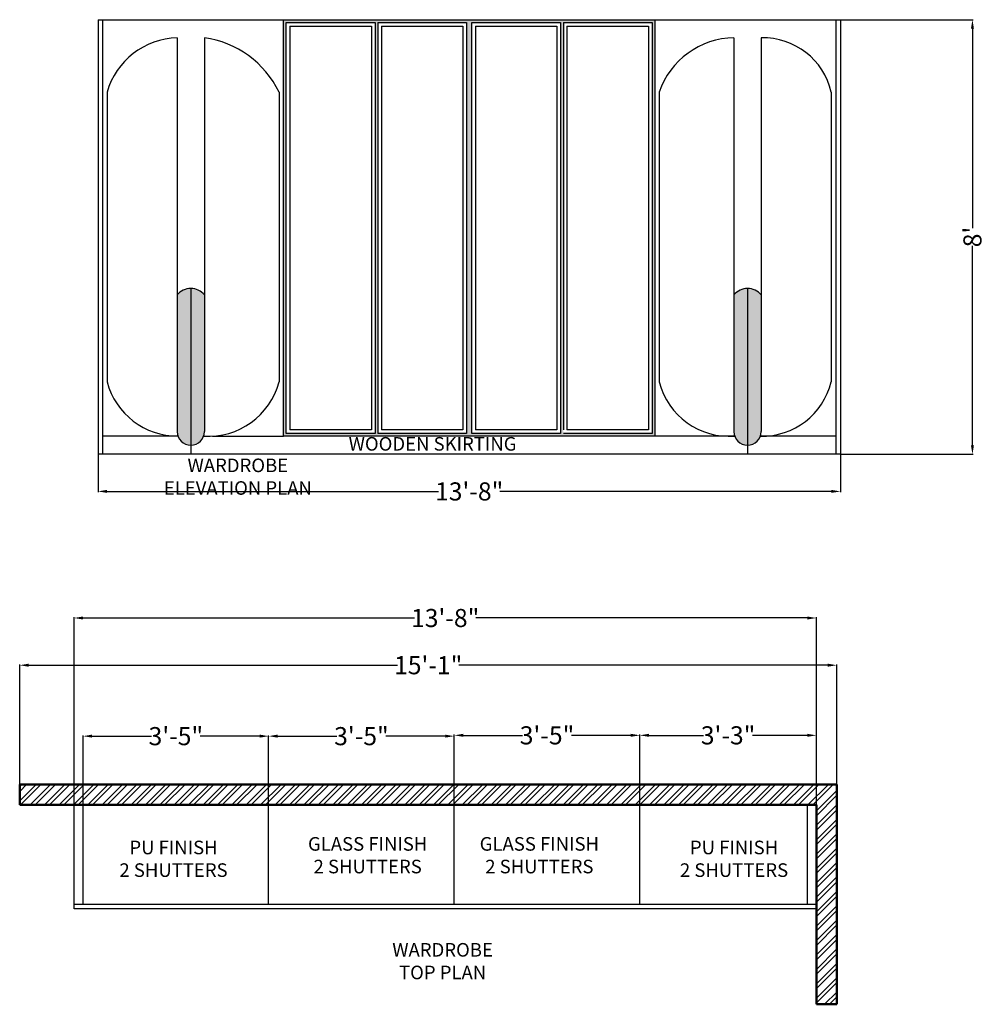
# Model space of a CAD drawing. Units: inches. Extents: x 210 to 423, y 38 to 255.
import ezdxf

# ---------------------------------------------------------------- set-up
doc = ezdxf.new("R2010")
doc.units = ezdxf.units.IN
doc.header["$MEASUREMENT"] = 0
for name, color, linetype, lineweight in [('A-ANNO-DIMS', 2, 'Continuous', 18), ('A-ANNO-TEXT', 7, 'Continuous', 18), ('A-FURN', 7, 'Continuous', 25), ('A-FURN-PATT', 42, 'Continuous', 13), ('A-WALL', 1, 'Continuous', 50), ('A-WALL-PATT', 8, 'Continuous', 13)]:
    doc.layers.add(name, color=color, linetype=linetype, lineweight=lineweight)
doc.styles.get("Standard").update_dxf_attribs({"font": 'arial.ttf'})
doc.dimstyles.get("Standard").update_dxf_attribs({"dimtxt": 4, "dimasz": 2, "dimexe": 0.18, "dimexo": 0.0625, "dimgap": 0.09, "dimtad": 0, "dimdec": 0, "dimzin": 0, "dimdsep": 46, "dimlunit": 4, "dimtxsty": 'Standard', "dimcen": 0.09, "dimadec": 0, "dimazin": 0, "dimtfac": 1, "dimtdec": 0, "dimtofl": 0, "dimtmove": 0, "dimatfit": 3, "dimfxl": 1, "dimtolj": 1, "dimtzin": 0, "dimarcsym": 0})

# ---------------------------------------------------------------- blocks, each defined once
blk = doc.blocks.new('*D1')
at = {"layer": 'A-ANNO-DIMS', "color": 0, "lineweight": -2, "transparency": 16777216}
for p, q in [((227.24, 159.18), (227.24, 150.86)), ((391.24, 159.18), (391.24, 150.86)), ((229.24, 151.04), (302.47, 151.04)), ((389.24, 151.04), (316.01, 151.04))]:
    blk.add_line(p, q, dxfattribs=at)
at = {"layer": 'A-ANNO-DIMS', "color": 0, "transparency": 16777216}
for points in [[(229.24, 151.38), (229.24, 150.71), (227.24, 151.04)], [(389.24, 151.38), (389.24, 150.71), (391.24, 151.04)]]:
    blk.add_solid(points, dxfattribs=at)
at = {"layer": 'Defpoints', "color": 0, "transparency": 16777216}
for p in [(227.24, 159.24), (391.24, 159.24), (227.24, 151.04)]:
    blk.add_point(p, dxfattribs=at)
at = {"layer": 'A-ANNO-DIMS', "color": 0, "transparency": 16777216, "insert": (309.24, 151.04), "char_height": 4, "attachment_point": 5}
blk.add_mtext('\\A1;13\'-8"', dxfattribs=at)
blk = doc.blocks.new('*D2')
at = {"layer": 'A-ANNO-DIMS', "color": 0, "lineweight": -2, "transparency": 16777216}
for p, q in [((391.3, 255.24), (420.6, 255.24)), ((420.42, 253.24), (420.42, 209.18)), ((420.42, 161.24), (420.42, 205.31)), ((391.3, 159.24), (420.6, 159.24))]:
    blk.add_line(p, q, dxfattribs=at)
at = {"layer": 'A-ANNO-DIMS', "color": 0, "transparency": 16777216}
for points in [[(420.08, 253.24), (420.75, 253.24), (420.42, 255.24)], [(420.08, 161.24), (420.75, 161.24), (420.42, 159.24)]]:
    blk.add_solid(points, dxfattribs=at)
at = {"layer": 'Defpoints', "color": 0, "transparency": 16777216}
for p in [(391.24, 255.24), (420.42, 255.24), (391.24, 159.24)]:
    blk.add_point(p, dxfattribs=at)
at = {"layer": 'A-ANNO-DIMS', "color": 0, "transparency": 16777216, "insert": (420.42, 207.24), "char_height": 4, "attachment_point": 5, "rotation": 90}
blk.add_mtext("\\A1;8'", dxfattribs=at)
blk = doc.blocks.new('*D3')
at = {"layer": 'A-ANNO-DIMS', "color": 0, "lineweight": -2, "transparency": 16777216}
for p, q in [((223.94, 81.86), (223.94, 97.16)), ((225.94, 96.98), (239.03, 96.98)), ((262.94, 96.98), (249.84, 96.98)), ((264.94, 81.86), (264.94, 97.16))]:
    blk.add_line(p, q, dxfattribs=at)
at = {"layer": 'A-ANNO-DIMS', "color": 0, "transparency": 16777216}
for points in [[(225.94, 97.32), (225.94, 96.65), (223.94, 96.98)], [(262.94, 97.32), (262.94, 96.65), (264.94, 96.98)]]:
    blk.add_solid(points, dxfattribs=at)
at = {"layer": 'Defpoints', "color": 0, "transparency": 16777216}
for p in [(264.94, 96.98), (223.94, 81.8), (264.94, 81.8)]:
    blk.add_point(p, dxfattribs=at)
at = {"layer": 'A-ANNO-DIMS', "color": 0, "transparency": 16777216, "insert": (244.44, 96.98), "char_height": 4, "attachment_point": 5}
blk.add_mtext('\\A1;3\'-5"', dxfattribs=at)
blk = doc.blocks.new('*D4')
at = {"layer": 'A-ANNO-DIMS', "color": 0, "lineweight": -2, "transparency": 16777216}
for p, q in [((264.94, 81.86), (264.94, 97.16)), ((266.94, 96.98), (280.03, 96.98)), ((303.94, 96.98), (290.84, 96.98)), ((305.94, 81.86), (305.94, 97.16))]:
    blk.add_line(p, q, dxfattribs=at)
at = {"layer": 'A-ANNO-DIMS', "color": 0, "transparency": 16777216}
for points in [[(266.94, 97.32), (266.94, 96.65), (264.94, 96.98)], [(303.94, 97.32), (303.94, 96.65), (305.94, 96.98)]]:
    blk.add_solid(points, dxfattribs=at)
at = {"layer": 'Defpoints', "color": 0, "transparency": 16777216}
for p in [(305.94, 96.98), (264.94, 81.8), (305.94, 81.8)]:
    blk.add_point(p, dxfattribs=at)
at = {"layer": 'A-ANNO-DIMS', "color": 0, "transparency": 16777216, "insert": (285.44, 96.98), "char_height": 4, "attachment_point": 5}
blk.add_mtext('\\A1;3\'-5"', dxfattribs=at)
blk = doc.blocks.new('*D5')
at = {"layer": 'A-ANNO-DIMS', "color": 0, "lineweight": -2, "transparency": 16777216}
for p, q in [((305.94, 81.86), (305.94, 97.34)), ((307.94, 97.16), (321.03, 97.16)), ((344.94, 97.16), (331.84, 97.16)), ((346.94, 81.86), (346.94, 97.34))]:
    blk.add_line(p, q, dxfattribs=at)
at = {"layer": 'A-ANNO-DIMS', "color": 0, "transparency": 16777216}
for points in [[(307.94, 97.5), (307.94, 96.83), (305.94, 97.16)], [(344.94, 97.5), (344.94, 96.83), (346.94, 97.16)]]:
    blk.add_solid(points, dxfattribs=at)
at = {"layer": 'Defpoints', "color": 0, "transparency": 16777216}
for p in [(346.94, 97.16), (305.94, 81.8), (346.94, 81.8)]:
    blk.add_point(p, dxfattribs=at)
at = {"layer": 'A-ANNO-DIMS', "color": 0, "transparency": 16777216, "insert": (326.44, 97.16), "char_height": 4, "attachment_point": 5}
blk.add_mtext('\\A1;3\'-5"', dxfattribs=at)
blk = doc.blocks.new('*D6')
at = {"layer": 'A-ANNO-DIMS', "color": 0, "lineweight": -2, "transparency": 16777216}
for p, q in [((346.94, 81.86), (346.94, 97.34)), ((348.94, 97.16), (361.03, 97.16)), ((383.94, 97.16), (371.84, 97.16)), ((385.94, 81.86), (385.94, 97.34))]:
    blk.add_line(p, q, dxfattribs=at)
at = {"layer": 'A-ANNO-DIMS', "color": 0, "transparency": 16777216}
for points in [[(348.94, 97.5), (348.94, 96.83), (346.94, 97.16)], [(383.94, 97.5), (383.94, 96.83), (385.94, 97.16)]]:
    blk.add_solid(points, dxfattribs=at)
at = {"layer": 'Defpoints', "color": 0, "transparency": 16777216}
for p in [(385.94, 97.16), (346.94, 81.8), (385.94, 81.8)]:
    blk.add_point(p, dxfattribs=at)
at = {"layer": 'A-ANNO-DIMS', "color": 0, "transparency": 16777216, "insert": (366.44, 97.16), "char_height": 4, "attachment_point": 5}
blk.add_mtext('\\A1;3\'-3"', dxfattribs=at)
blk = doc.blocks.new('*D7')
at = {"layer": 'A-ANNO-DIMS', "color": 0, "lineweight": -2, "transparency": 16777216}
for p, q in [((221.94, 58.86), (221.94, 123.26)), ((223.94, 123.08), (297.17, 123.08)), ((383.94, 123.08), (310.71, 123.08)), ((385.94, 58.86), (385.94, 123.26))]:
    blk.add_line(p, q, dxfattribs=at)
at = {"layer": 'A-ANNO-DIMS', "color": 0, "transparency": 16777216}
for points in [[(223.94, 123.41), (223.94, 122.74), (221.94, 123.08)], [(383.94, 123.41), (383.94, 122.74), (385.94, 123.08)]]:
    blk.add_solid(points, dxfattribs=at)
at = {"layer": 'Defpoints', "color": 0, "transparency": 16777216}
for p in [(221.94, 123.08), (221.94, 58.8), (385.94, 58.8)]:
    blk.add_point(p, dxfattribs=at)
at = {"layer": 'A-ANNO-DIMS', "color": 0, "transparency": 16777216, "insert": (303.94, 123.08), "char_height": 4, "attachment_point": 5}
blk.add_mtext('\\A1;13\'-8"', dxfattribs=at)
blk = doc.blocks.new('*D8')
at = {"layer": 'A-ANNO-DIMS', "color": 0, "lineweight": -2, "transparency": 16777216}
for p, q in [((209.94, 86.36), (209.94, 112.83)), ((211.94, 112.65), (293.42, 112.65)), ((388.44, 112.65), (306.96, 112.65)), ((390.44, 86.36), (390.44, 112.83))]:
    blk.add_line(p, q, dxfattribs=at)
at = {"layer": 'A-ANNO-DIMS', "color": 0, "transparency": 16777216}
for points in [[(211.94, 112.99), (211.94, 112.32), (209.94, 112.65)], [(388.44, 112.99), (388.44, 112.32), (390.44, 112.65)]]:
    blk.add_solid(points, dxfattribs=at)
at = {"layer": 'Defpoints', "color": 0, "transparency": 16777216}
for p in [(390.44, 112.65), (209.94, 86.3), (390.44, 86.3)]:
    blk.add_point(p, dxfattribs=at)
at = {"layer": 'A-ANNO-DIMS', "color": 0, "transparency": 16777216, "insert": (300.19, 112.65), "char_height": 4, "attachment_point": 5}
blk.add_mtext('\\A1;15\'-1"', dxfattribs=at)
blk = doc.blocks.new('GLASS-SHUTTER-PANEL')
for p, q in [((0, 89.2), (0, 0)), ((0, 89.2), (18, 89.2)), ((18, 89.2), (18, 0)), ((18, 0), (0, 0))]:
    blk.add_line(p, q)

msp = doc.modelspace()

# ---------------------------------------------------------------- hatches: boundary and pattern name
at = {"layer": 'A-FURN-PATT'}
h = msp.add_hatch(color=256, dxfattribs=at)
h.dxf.hatch_style = 1
h.paths.add_polyline_path([(350.24, 255.24), (309.24, 255.24), (268.24, 255.24), (268.24, 163.24), (350.24, 163.24)])
h.paths.add_polyline_path([(308.64, 163.84), (268.84, 163.84), (268.84, 254.64), (308.64, 254.64)], flags=16)
h.paths.add_polyline_path([(309.84, 254.64), (349.64, 254.64), (349.64, 163.84), (309.84, 163.84)], flags=16)
h.paths.add_polyline_path([(307.84, 253.84), (307.84, 164.64), (269.64, 164.64), (269.64, 253.84)], flags=0)
h.paths.add_polyline_path([(310.64, 253.84), (348.84, 253.84), (348.84, 164.64), (310.64, 164.64)], flags=0)
h = msp.add_hatch(color=256, dxfattribs=at)
h.dxf.hatch_style = 1
h.paths.add_polyline_path([(289.04, 254.64), (288.44, 254.64), (288.44, 163.84), (289.04, 163.84)])
h = msp.add_hatch(color=256, dxfattribs=at)
h.dxf.hatch_style = 1
h.paths.add_polyline_path([(330.04, 254.64), (329.44, 254.64), (329.44, 163.84), (330.04, 163.84)])
h = msp.add_hatch(color=256, dxfattribs=at)
h.dxf.hatch_style = 1
h.paths.add_polyline_path([(247.74, 195.86, 0.225589), (244.74, 194.43), (244.74, 164.25, 0.414214), (247.74, 161.25)])
h.paths.add_polyline_path([(250.74, 194.43, 0.225589), (247.74, 195.86), (247.74, 161.25, 0.414214), (250.74, 164.25)])
h.paths.add_polyline_path([(370.74, 195.86, 0.225589), (367.74, 194.43), (367.74, 164.25, 0.414214), (370.74, 161.25)])
h.paths.add_polyline_path([(373.74, 194.43, 0.225589), (370.74, 195.86), (370.74, 161.25, 0.414214), (373.74, 164.25)])
at = {"layer": 'A-WALL-PATT'}
h = msp.add_hatch(dxfattribs=at)
h.set_pattern_fill('ANSI32', color=256, scale=6)
h.paths.add_polyline_path([(390.44, 86.3), (385.94, 86.3), (209.94, 86.3), (209.94, 81.8), (385.94, 81.8), (385.94, 37.75), (390.44, 37.75)])

# ---------------------------------------------------------------- linework, layer by layer
at = {"layer": 'A-FURN'}
for p, q in [((227.24, 255.24), (227.24, 159.24)), ((227.24, 255.24), (268.24, 255.24)), ((228.24, 255.24), (228.24, 159.24)), ((288.44, 254.64), (288.44, 163.84)), ((289.04, 254.64), (289.04, 163.84)), ((329.44, 254.64), (329.44, 163.84)), ((330.04, 254.64), (330.04, 164.64)), ((350.24, 255.24), (391.24, 255.24)), ((390.24, 255.24), (390.24, 159.24)), ((391.24, 255.24), (391.24, 159.24)), ((288.44, 253.84), (288.44, 164.64)), ((244.74, 251.24), (244.74, 164.25)), ((250.74, 251.24), (250.74, 164.25)), ((367.74, 251.24), (367.74, 164.25)), ((373.74, 251.24), (373.74, 164.25)), ((229.24, 239.24), (229.24, 175.24)), ((267.24, 239.24), (267.24, 175.24)), ((351.24, 239.24), (351.24, 175.24)), ((389.24, 239.24), (389.24, 175.24)), ((247.74, 195.86), (247.74, 159.24)), ((370.74, 195.86), (370.74, 159.24)), ((244.74, 163.24), (228.24, 163.24)), ((252.51, 163.24), (268.24, 163.24)), ((367.74, 163.24), (268.24, 163.24)), ((390.24, 163.24), (373.74, 163.24)), ((391.24, 159.24), (227.24, 159.24)), ((221.94, 58.8), (221.94, 81.8)), ((221.94, 81.8), (385.94, 81.8)), ((223.94, 59.8), (223.94, 81.8)), ((264.94, 59.8), (264.94, 81.8)), ((305.94, 59.8), (305.94, 81.8)), ((346.94, 59.8), (346.94, 81.8)), ((383.94, 81.8), (383.94, 59.8)), ((385.94, 81.8), (385.94, 58.8)), ((385.94, 59.8), (221.94, 59.8)), ((385.94, 58.8), (221.94, 58.8))]:
    msp.add_line(p, q, dxfattribs=at)
msp.add_lwpolyline([(309.24, 255.24), (350.24, 255.24), (350.24, 163.24), (268.24, 163.24), (268.24, 255.24)], close=True, dxfattribs=at)
for points in [[(288.44, 163.84), (268.84, 163.84), (268.84, 254.64), (288.44, 254.64)], [(289.04, 254.64), (308.64, 254.64), (308.64, 163.84), (289.04, 163.84)], [(329.44, 163.84), (309.84, 163.84), (309.84, 254.64), (329.44, 254.64)], [(330.04, 254.64), (349.64, 254.64), (349.64, 163.84), (330.04, 163.84)]]:
    msp.add_lwpolyline(points, dxfattribs=at)
for centre, radius, start, end in [((245.15, 234.7), 16.54, 91.4162, 164.0774), ((247.74, 229.77), 21.68, 25.9001, 82.0451), ((367.98, 233.57), 17.68, 90.7845, 161.2702), ((374.13, 235.74), 15.51, 13.0673, 91.4391), ((247.74, 191.99), 3.87, 39.1501, 140.8499), ((370.74, 191.99), 3.87, 39.1501, 140.8499), ((244.92, 179.49), 16.25, 195.1455, 269.9775), ((251.63, 179.37), 16.15, 266.2461, 345.2015), ((366.67, 179.11), 15.9, 194.0717, 274.4879), ((373.94, 179), 15.75, 268.6454, 346.2176), ((247.74, 164.25), 3, 180, 0), ((247.74, 164.25), 3, 180, 0), ((370.74, 164.25), 3, 180, 0)]:
    msp.add_arc(centre, radius, start, end, dxfattribs=at)
at = {"layer": 'A-WALL'}
for p, q in [((209.94, 81.8), (209.94, 86.3)), ((209.94, 86.3), (385.94, 86.3)), ((385.94, 86.3), (390.44, 86.3)), ((390.44, 86.3), (390.44, 37.75)), ((385.94, 81.8), (209.94, 81.8)), ((385.94, 37.75), (385.94, 81.8)), ((390.44, 37.75), (385.94, 37.75))]:
    msp.add_line(p, q, dxfattribs=at)

# ---------------------------------------------------------------- block references
at = {"layer": 'A-FURN'}
for p in [(269.64, 164.64), (289.84, 164.64), (310.64, 164.64), (330.84, 164.64)]:
    msp.add_blockref('GLASS-SHUTTER-PANEL', p, dxfattribs=at)

# ---------------------------------------------------------------- texts
at = {"layer": 'A-ANNO-TEXT', "char_height": 3, "attachment_point": 1}
for s, width, insert in [('\\pxqc;WOODEN SKIRTING', 50.0034, (276.15, 163.05)), ('\\pxqc;WARDROBE\\PELEVATION PLAN', 41.3697, (237.45, 158.3)), ('\\pxqc;GLASS FINISH \\P2 SHUTTERS', 31.9464, (270.84, 74.68)), ('\\pxqc;GLASS FINISH \\P2 SHUTTERS', 31.9464, (308.77, 74.68)), ('\\pxqc;PU FINISH \\P2 SHUTTERS', 32.1832, (227.83, 73.89)), ('\\pxqc;PU FINISH \\P2 SHUTTERS', 32.1832, (351.66, 73.89)), ('\\pxqc;WARDROBE \\PTOP PLAN', 73.2103, (266.76, 51.28))]:
    msp.add_mtext_dynamic_manual_height_columns(s, width=width, gutter_width=15, heights=[0], dxfattribs=dict(at, insert=insert))

# ---------------------------------------------------------------- dimensions: what is measured, and where the dimension line sits
at = {"layer": 'A-ANNO-DIMS'}
dim = msp.add_linear_dim(base=(420.42, 255.24), p1=(391.24, 159.24), p2=(391.24, 255.24), angle=90, dimstyle='Standard', override={"dimclrd": 0, "dimclre": 0, "dimclrt": 0}, dxfattribs=at)
dim.commit()
dim.dimension.update_dxf_attribs({"geometry": '*D2', "text_midpoint": (420.42, 207.24)})
for base, p1, p2, picture, middle in [((227.24, 151.04), (391.24, 159.24), (227.24, 159.24), '*D1', (309.24, 151.04)), ((221.94, 123.08), (385.94, 58.8), (221.94, 58.8), '*D7', (303.94, 123.08)), ((390.43968071, 112.65184868), (209.93968071, 86.30043895), (390.43968071, 86.30043895), '*D8', (300.18968071, 112.65184868)), ((264.94, 96.98), (223.94, 81.8), (264.94, 81.8), '*D3', (244.44, 96.98)), ((305.94, 96.98), (264.94, 81.8), (305.94, 81.8), '*D4', (285.44, 96.98)), ((346.94, 97.16), (305.94, 81.8), (346.94, 81.8), '*D5', (326.44, 97.16)), ((385.94, 97.16), (346.94, 81.8), (385.94, 81.8), '*D6', (366.44, 97.16))]:
    dim = msp.add_linear_dim(base=base, p1=p1, p2=p2, dimstyle='Standard', override={"dimclrd": 0, "dimclre": 0, "dimclrt": 0}, dxfattribs=at)
    dim.commit()
    dim.dimension.update_dxf_attribs({"geometry": picture, "text_midpoint": middle})

doc.saveas('drawing.dxf')
